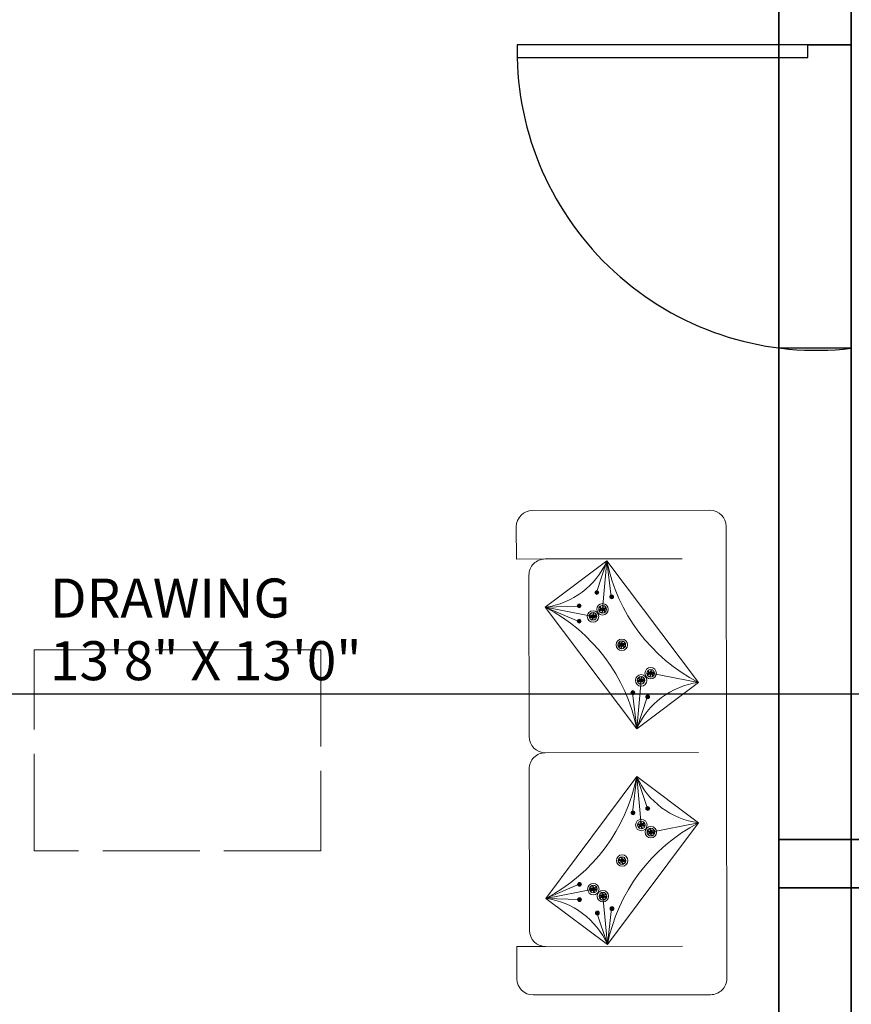
# Model space of a CAD drawing. Units: inches. Extents: x -61 to 1599, y -1316 to 257.
# Tile 30 of 204: x 442 to 545, y -912 to -790. Entities that reach past the tile are written whole.
import ezdxf

# ---------------------------------------------------------------- set-up
doc = ezdxf.new("R2010")
doc.units = ezdxf.units.IN
doc.header["$MEASUREMENT"] = 0
doc.linetypes.add('ACAD_ISO02W100', pattern=[15, 12, -3])
for name, color, linetype, lineweight in [('A-ANNO-DIMS', 2, 'Continuous', 18), ('A-AREA-IDEN', 1, 'Continuous', 18), ('A-FURN-LOW', 83, 'ACAD_ISO02W100', 18), ('A-WALL-JAMB', 4, 'ACAD_ISO02W100', 25), ('DOORS', 2, 'Continuous', 25), ('FURNITURE', 83, 'Continuous', 18), ('WALLS', 4, 'Continuous', 35)]:
    doc.layers.add(name, color=color, linetype=linetype, lineweight=lineweight)
doc.layers.add('FUR', color=83, linetype='Continuous')
doc.styles.get("Standard").update_dxf_attribs({"font": 'arial.ttf'})
doc.dimstyles.get("Standard").update_dxf_attribs({"dimtxt": 0.18, "dimasz": 0.18, "dimexe": 0.18, "dimexo": 0.0625, "dimgap": 0.09, "dimtad": 0, "dimtih": 1, "dimtoh": 1, "dimdec": 0, "dimzin": 0, "dimdsep": 46, "dimlunit": 3, "dimtxsty": 'Standard', "dimcen": 0.09, "dimadec": 0, "dimazin": 0, "dimtfac": 1, "dimtdec": 0, "dimtofl": 0, "dimtmove": 0, "dimatfit": 3, "dimfxl": 1, "dimtolj": 1, "dimtzin": 0, "dimarcsym": 0})

# ---------------------------------------------------------------- blocks, each defined once
blk = doc.blocks.new('*U382')
at = {"layer": 'FUR'}
blk.add_open_spline([(0.01, 0.24), (-0.09, 0.14), (-0.29, -0.05), (0.22, -0.05), (0.07, -0.19), (0.01, -0.24)], degree=3, knots=[0, 0, 0, 0, 0.2846533, 0.5662105, 0.736751, 0.736751, 0.736751, 0.736751], dxfattribs=at)
blk = doc.blocks.new('*U383')
at = {"layer": 'FURNITURE', "transparency": 16777216}
for p, rotation in [((662.52, -238.49), 60), ((662.53, -238.73), 120), ((662.74, -238.83), 180), ((662.93, -238.46), 300), ((662.94, -238.7), 240)]:
    blk.add_blockref('*U382', p, dxfattribs=dict(at, rotation=rotation))
blk.add_blockref('*U382', (662.72, -238.36), dxfattribs=at)
blk = doc.blocks.new('*U394')
at = {"layer": 'FUR'}
blk.add_open_spline([(0.01, 0.24), (-0.09, 0.14), (-0.29, -0.05), (0.22, -0.05), (0.07, -0.19), (0.01, -0.24)], degree=3, knots=[0, 0, 0, 0, 0.2846533, 0.5662105, 0.736751, 0.736751, 0.736751, 0.736751], dxfattribs=at)
blk = doc.blocks.new('*U411')
at = {"layer": 'FURNITURE', "transparency": 16777216}
for p, rotation in [((662.52, -238.49), 60), ((662.53, -238.73), 120), ((662.74, -238.83), 180), ((662.93, -238.46), 300), ((662.94, -238.7), 240)]:
    blk.add_blockref('*U394', p, dxfattribs=dict(at, rotation=rotation))
blk.add_blockref('*U394', (662.72, -238.36), dxfattribs=at)
blk = doc.blocks.new('*U384')
at = {"layer": 'FUR'}
blk.add_open_spline([(0, 0.08), (-0.03, 0.05), (-0.1, -0.02), (0.08, -0.02), (0.02, -0.06), (0, -0.08)], degree=3, knots=[0, 0, 0, 0, 0.0954578, 0.1898773, 0.2470677, 0.2470677, 0.2470677, 0.2470677], dxfattribs=at)
blk = doc.blocks.new('*U385')
at = {"layer": 'FURNITURE', "transparency": 16777216}
for p, rotation in [((222.17, -79.98), 60), ((222.18, -80.06), 120), ((222.31, -79.97), 300), ((222.25, -80.09), 180), ((222.32, -80.05), 240)]:
    blk.add_blockref('*U384', p, dxfattribs=dict(at, rotation=rotation))
blk.add_blockref('*U384', (222.24, -79.93), dxfattribs=at)
blk = doc.blocks.new('*U386')
at = {"layer": 'FUR'}
blk.add_open_spline([(0, 0.08), (-0.03, 0.05), (-0.1, -0.02), (0.08, -0.02), (0.02, -0.06), (0, -0.08)], degree=3, knots=[0, 0, 0, 0, 0.0954578, 0.1898773, 0.2470677, 0.2470677, 0.2470677, 0.2470677], dxfattribs=at)
blk = doc.blocks.new('*U387')
at = {"layer": 'FURNITURE', "transparency": 16777216}
for p, rotation in [((222.17, -79.98), 60), ((222.18, -80.06), 120), ((222.31, -79.97), 300), ((222.25, -80.09), 180), ((222.32, -80.05), 240)]:
    blk.add_blockref('*U386', p, dxfattribs=dict(at, rotation=rotation))
blk.add_blockref('*U386', (222.24, -79.93), dxfattribs=at)
blk = doc.blocks.new('*U388')
at = {"layer": 'FUR'}
blk.add_open_spline([(0, 0.08), (-0.03, 0.05), (-0.1, -0.02), (0.08, -0.02), (0.02, -0.06), (0, -0.08)], degree=3, knots=[0, 0, 0, 0, 0.0954578, 0.1898773, 0.2470677, 0.2470677, 0.2470677, 0.2470677], dxfattribs=at)
blk = doc.blocks.new('*U389')
at = {"layer": 'FURNITURE', "transparency": 16777216}
for p, rotation in [((222.17, -79.98), 60), ((222.18, -80.06), 120), ((222.31, -79.97), 300), ((222.25, -80.09), 180), ((222.32, -80.05), 240)]:
    blk.add_blockref('*U388', p, dxfattribs=dict(at, rotation=rotation))
blk.add_blockref('*U388', (222.24, -79.93), dxfattribs=at)
blk = doc.blocks.new('*U390')
at = {"layer": 'FUR'}
blk.add_open_spline([(0, 0.08), (-0.03, 0.05), (-0.1, -0.02), (0.08, -0.02), (0.02, -0.06), (0, -0.08)], degree=3, knots=[0, 0, 0, 0, 0.0954578, 0.1898773, 0.2470677, 0.2470677, 0.2470677, 0.2470677], dxfattribs=at)
blk = doc.blocks.new('*U391')
at = {"layer": 'FURNITURE', "transparency": 16777216}
for p, rotation in [((222.17, -79.98), 60), ((222.18, -80.06), 120), ((222.31, -79.97), 300), ((222.25, -80.09), 180), ((222.32, -80.05), 240)]:
    blk.add_blockref('*U390', p, dxfattribs=dict(at, rotation=rotation))
blk.add_blockref('*U390', (222.24, -79.93), dxfattribs=at)
blk = doc.blocks.new('*U392')
at = {"layer": 'FUR'}
blk.add_open_spline([(0, 0.08), (-0.03, 0.05), (-0.1, -0.02), (0.08, -0.02), (0.02, -0.06), (0, -0.08)], degree=3, knots=[0, 0, 0, 0, 0.0954578, 0.1898773, 0.2470677, 0.2470677, 0.2470677, 0.2470677], dxfattribs=at)
blk = doc.blocks.new('*U413')
at = {"layer": 'FURNITURE', "transparency": 16777216}
for p, rotation in [((222.17, -79.98), 60), ((222.18, -80.06), 120), ((222.31, -79.97), 300), ((222.25, -80.09), 180), ((222.32, -80.05), 240)]:
    blk.add_blockref('*U392', p, dxfattribs=dict(at, rotation=rotation))
blk.add_blockref('*U392', (222.24, -79.93), dxfattribs=at)
blk = doc.blocks.new('*U414')
at = {"layer": 'FUR'}
blk.add_open_spline([(0, 0.08), (-0.03, 0.05), (-0.1, -0.02), (0.08, -0.02), (0.02, -0.06), (0, -0.08)], degree=3, knots=[0, 0, 0, 0, 0.0954578, 0.1898773, 0.2470677, 0.2470677, 0.2470677, 0.2470677], dxfattribs=at)
blk = doc.blocks.new('*U415')
at = {"layer": 'FURNITURE', "transparency": 16777216}
for p, rotation in [((222.17, -79.98), 60), ((222.18, -80.06), 120), ((222.31, -79.97), 300), ((222.25, -80.09), 180), ((222.32, -80.05), 240)]:
    blk.add_blockref('*U414', p, dxfattribs=dict(at, rotation=rotation))
blk.add_blockref('*U414', (222.24, -79.93), dxfattribs=at)
blk = doc.blocks.new('*U416')
at = {"layer": 'FUR'}
blk.add_open_spline([(0.01, 0.24), (-0.09, 0.14), (-0.29, -0.05), (0.22, -0.05), (0.07, -0.19), (0.01, -0.24)], degree=3, knots=[0, 0, 0, 0, 0.2846533, 0.5662105, 0.736751, 0.736751, 0.736751, 0.736751], dxfattribs=at)
blk = doc.blocks.new('*U417')
at = {"layer": 'FURNITURE', "transparency": 16777216}
for p, rotation in [((662.52, -238.49), 60), ((662.53, -238.73), 120), ((662.74, -238.83), 180), ((662.93, -238.46), 300), ((662.94, -238.7), 240)]:
    blk.add_blockref('*U416', p, dxfattribs=dict(at, rotation=rotation))
blk.add_blockref('*U416', (662.72, -238.36), dxfattribs=at)
blk = doc.blocks.new('*U418')
at = {"layer": 'FUR'}
blk.add_open_spline([(0.01, 0.24), (-0.09, 0.14), (-0.29, -0.05), (0.22, -0.05), (0.07, -0.19), (0.01, -0.24)], degree=3, knots=[0, 0, 0, 0, 0.2846533, 0.5662105, 0.736751, 0.736751, 0.736751, 0.736751], dxfattribs=at)
blk = doc.blocks.new('*U381')
at = {"layer": 'FURNITURE', "transparency": 16777216}
for p, rotation in [((662.52, -238.49), 60), ((662.53, -238.73), 120), ((662.74, -238.83), 180), ((662.93, -238.46), 300), ((662.94, -238.7), 240)]:
    blk.add_blockref('*U418', p, dxfattribs=dict(at, rotation=rotation))
blk.add_blockref('*U418', (662.72, -238.36), dxfattribs=at)
blk = doc.blocks.new('*U393')
at = {"layer": 'FUR'}
blk.add_open_spline([(0.01, 0.24), (-0.09, 0.14), (-0.29, -0.05), (0.22, -0.05), (0.07, -0.19), (0.01, -0.24)], degree=3, knots=[0, 0, 0, 0, 0.2846533, 0.5662105, 0.736751, 0.736751, 0.736751, 0.736751], dxfattribs=at)
blk = doc.blocks.new('*U412')
at = {"layer": 'FURNITURE', "transparency": 16777216}
for p, rotation in [((662.52, -238.49), 60), ((662.53, -238.73), 120), ((662.74, -238.83), 180), ((662.93, -238.46), 300), ((662.94, -238.7), 240)]:
    blk.add_blockref('*U393', p, dxfattribs=dict(at, rotation=rotation))
blk.add_blockref('*U393', (662.72, -238.36), dxfattribs=at)
blk = doc.blocks.new('*U379')
at = {"layer": 'FUR'}
blk.add_open_spline([(0.01, 0.24), (-0.09, 0.14), (-0.29, -0.05), (0.22, -0.05), (0.07, -0.19), (0.01, -0.24)], degree=3, knots=[0, 0, 0, 0, 0.2846533, 0.5662105, 0.736751, 0.736751, 0.736751, 0.736751], dxfattribs=at)
blk = doc.blocks.new('*U380')
at = {"layer": 'FURNITURE', "transparency": 16777216}
for p, rotation in [((662.52, -238.49), 60), ((662.53, -238.73), 120), ((662.74, -238.83), 180), ((662.93, -238.46), 300), ((662.94, -238.7), 240)]:
    blk.add_blockref('*U379', p, dxfattribs=dict(at, rotation=rotation))
blk.add_blockref('*U379', (662.72, -238.36), dxfattribs=at)
blk = doc.blocks.new('*U410')
at = {"layer": 'FUR'}
blk.add_open_spline([(0.01, 0.24), (-0.09, 0.14), (-0.29, -0.05), (0.22, -0.05), (0.07, -0.19), (0.01, -0.24)], degree=3, knots=[0, 0, 0, 0, 0.2846533, 0.5662105, 0.736751, 0.736751, 0.736751, 0.736751], dxfattribs=at)
blk = doc.blocks.new('*U395')
at = {"layer": 'FURNITURE', "transparency": 16777216}
for p, rotation in [((662.52, -238.49), 60), ((662.53, -238.73), 120), ((662.74, -238.83), 180), ((662.93, -238.46), 300), ((662.94, -238.7), 240)]:
    blk.add_blockref('*U410', p, dxfattribs=dict(at, rotation=rotation))
blk.add_blockref('*U410', (662.72, -238.36), dxfattribs=at)
blk = doc.blocks.new('*U400')
at = {"layer": 'FUR'}
blk.add_open_spline([(0, 0.08), (-0.03, 0.05), (-0.1, -0.02), (0.08, -0.02), (0.02, -0.06), (0, -0.08)], degree=3, knots=[0, 0, 0, 0, 0.0954578, 0.1898773, 0.2470677, 0.2470677, 0.2470677, 0.2470677], dxfattribs=at)
blk = doc.blocks.new('*U401')
at = {"layer": 'FURNITURE', "transparency": 16777216}
for p, rotation in [((222.17, -79.98), 60), ((222.18, -80.06), 120), ((222.31, -79.97), 300), ((222.25, -80.09), 180), ((222.32, -80.05), 240)]:
    blk.add_blockref('*U400', p, dxfattribs=dict(at, rotation=rotation))
blk.add_blockref('*U400', (222.24, -79.93), dxfattribs=at)
blk = doc.blocks.new('*U402')
at = {"layer": 'FUR'}
blk.add_open_spline([(0, 0.08), (-0.03, 0.05), (-0.1, -0.02), (0.08, -0.02), (0.02, -0.06), (0, -0.08)], degree=3, knots=[0, 0, 0, 0, 0.0954578, 0.1898773, 0.2470677, 0.2470677, 0.2470677, 0.2470677], dxfattribs=at)
blk = doc.blocks.new('*U403')
at = {"layer": 'FURNITURE', "transparency": 16777216}
for p, rotation in [((222.17, -79.98), 60), ((222.18, -80.06), 120), ((222.31, -79.97), 300), ((222.25, -80.09), 180), ((222.32, -80.05), 240)]:
    blk.add_blockref('*U402', p, dxfattribs=dict(at, rotation=rotation))
blk.add_blockref('*U402', (222.24, -79.93), dxfattribs=at)
blk = doc.blocks.new('*U404')
at = {"layer": 'FUR'}
blk.add_open_spline([(0, 0.08), (-0.03, 0.05), (-0.1, -0.02), (0.08, -0.02), (0.02, -0.06), (0, -0.08)], degree=3, knots=[0, 0, 0, 0, 0.0954578, 0.1898773, 0.2470677, 0.2470677, 0.2470677, 0.2470677], dxfattribs=at)
blk = doc.blocks.new('*U405')
at = {"layer": 'FURNITURE', "transparency": 16777216}
for p, rotation in [((222.17, -79.98), 60), ((222.18, -80.06), 120), ((222.31, -79.97), 300), ((222.25, -80.09), 180), ((222.32, -80.05), 240)]:
    blk.add_blockref('*U404', p, dxfattribs=dict(at, rotation=rotation))
blk.add_blockref('*U404', (222.24, -79.93), dxfattribs=at)
blk = doc.blocks.new('*U406')
at = {"layer": 'FUR'}
blk.add_open_spline([(0, 0.08), (-0.03, 0.05), (-0.1, -0.02), (0.08, -0.02), (0.02, -0.06), (0, -0.08)], degree=3, knots=[0, 0, 0, 0, 0.0954578, 0.1898773, 0.2470677, 0.2470677, 0.2470677, 0.2470677], dxfattribs=at)
blk = doc.blocks.new('*U407')
at = {"layer": 'FURNITURE', "transparency": 16777216}
for p, rotation in [((222.17, -79.98), 60), ((222.18, -80.06), 120), ((222.31, -79.97), 300), ((222.25, -80.09), 180), ((222.32, -80.05), 240)]:
    blk.add_blockref('*U406', p, dxfattribs=dict(at, rotation=rotation))
blk.add_blockref('*U406', (222.24, -79.93), dxfattribs=at)
blk = doc.blocks.new('*U408')
at = {"layer": 'FUR'}
blk.add_open_spline([(0, 0.08), (-0.03, 0.05), (-0.1, -0.02), (0.08, -0.02), (0.02, -0.06), (0, -0.08)], degree=3, knots=[0, 0, 0, 0, 0.0954578, 0.1898773, 0.2470677, 0.2470677, 0.2470677, 0.2470677], dxfattribs=at)
blk = doc.blocks.new('*U397')
at = {"layer": 'FURNITURE', "transparency": 16777216}
for p, rotation in [((222.17, -79.98), 60), ((222.18, -80.06), 120), ((222.31, -79.97), 300), ((222.25, -80.09), 180), ((222.32, -80.05), 240)]:
    blk.add_blockref('*U408', p, dxfattribs=dict(at, rotation=rotation))
blk.add_blockref('*U408', (222.24, -79.93), dxfattribs=at)
blk = doc.blocks.new('*U398')
at = {"layer": 'FUR'}
blk.add_open_spline([(0, 0.08), (-0.03, 0.05), (-0.1, -0.02), (0.08, -0.02), (0.02, -0.06), (0, -0.08)], degree=3, knots=[0, 0, 0, 0, 0.0954578, 0.1898773, 0.2470677, 0.2470677, 0.2470677, 0.2470677], dxfattribs=at)
blk = doc.blocks.new('*U399')
at = {"layer": 'FURNITURE', "transparency": 16777216}
for p, rotation in [((222.17, -79.98), 60), ((222.18, -80.06), 120), ((222.31, -79.97), 300), ((222.25, -80.09), 180), ((222.32, -80.05), 240)]:
    blk.add_blockref('*U398', p, dxfattribs=dict(at, rotation=rotation))
blk.add_blockref('*U398', (222.24, -79.93), dxfattribs=at)
blk = doc.blocks.new('*U375')
at = {"layer": 'FUR'}
blk.add_open_spline([(0.01, 0.24), (-0.09, 0.14), (-0.29, -0.05), (0.22, -0.05), (0.07, -0.19), (0.01, -0.24)], degree=3, knots=[0, 0, 0, 0, 0.2846533, 0.5662105, 0.736751, 0.736751, 0.736751, 0.736751], dxfattribs=at)
blk = doc.blocks.new('*U376')
at = {"layer": 'FURNITURE', "transparency": 16777216}
for p, rotation in [((662.52, -238.49), 60), ((662.53, -238.73), 120), ((662.74, -238.83), 180), ((662.93, -238.46), 300), ((662.94, -238.7), 240)]:
    blk.add_blockref('*U375', p, dxfattribs=dict(at, rotation=rotation))
blk.add_blockref('*U375', (662.72, -238.36), dxfattribs=at)
blk = doc.blocks.new('*U377')
at = {"layer": 'FUR'}
blk.add_open_spline([(0.01, 0.24), (-0.09, 0.14), (-0.29, -0.05), (0.22, -0.05), (0.07, -0.19), (0.01, -0.24)], degree=3, knots=[0, 0, 0, 0, 0.2846533, 0.5662105, 0.736751, 0.736751, 0.736751, 0.736751], dxfattribs=at)
blk = doc.blocks.new('*U378')
at = {"layer": 'FURNITURE', "transparency": 16777216}
for p, rotation in [((662.52, -238.49), 60), ((662.53, -238.73), 120), ((662.74, -238.83), 180), ((662.93, -238.46), 300), ((662.94, -238.7), 240)]:
    blk.add_blockref('*U377', p, dxfattribs=dict(at, rotation=rotation))
blk.add_blockref('*U377', (662.72, -238.36), dxfattribs=at)
blk = doc.blocks.new('*U409')
at = {"layer": 'FUR'}
blk.add_open_spline([(0.01, 0.24), (-0.09, 0.14), (-0.29, -0.05), (0.22, -0.05), (0.07, -0.19), (0.01, -0.24)], degree=3, knots=[0, 0, 0, 0, 0.2846533, 0.5662105, 0.736751, 0.736751, 0.736751, 0.736751], dxfattribs=at)
blk = doc.blocks.new('*U396')
at = {"layer": 'FURNITURE', "transparency": 16777216}
for p, rotation in [((662.52, -238.49), 60), ((662.53, -238.73), 120), ((662.74, -238.83), 180), ((662.93, -238.46), 300), ((662.94, -238.7), 240)]:
    blk.add_blockref('*U409', p, dxfattribs=dict(at, rotation=rotation))
blk.add_blockref('*U409', (662.72, -238.36), dxfattribs=at)
blk = doc.blocks.new('DOOR-SWING-36')
blk.add_line((0, 0), (0, -5.4))
blk.add_lwpolyline([(0, 0), (0, 36), (-1.57, 36), (-1.57, 0)], close=True)
blk.add_arc((-0.74, -1.08), 37.09, 91.2913, 186.6905)
blk = doc.blocks.new('*D696')
at = {"layer": 'A-ANNO-DIMS', "color": 0, "lineweight": -2, "transparency": 16777216}
for p, q in [((690.64, -873.17), (-61.08, -873.17)), ((-60.9, -873.35), (-60.9, -1025.8)), ((-60.9, -1178.61), (-60.9, -1026.16)), ((690.64, -1178.79), (-61.08, -1178.79))]:
    blk.add_line(p, q, dxfattribs=at)
at = {"layer": 'A-ANNO-DIMS', "color": 0, "transparency": 16777216}
for points in [[(-60.93, -873.35), (-60.87, -873.35), (-60.9, -873.17)], [(-60.93, -1178.61), (-60.87, -1178.61), (-60.9, -1178.79)]]:
    blk.add_solid(points, dxfattribs=at)
at = {"layer": 'DEFPOINTS', "color": 0, "transparency": 16777216}
for p in [(-60.9, -873.17), (690.7, -873.17), (690.7, -1178.79)]:
    blk.add_point(p, dxfattribs=at)
at = {"layer": 'A-ANNO-DIMS', "color": 0, "transparency": 16777216, "insert": (-60.9, -1025.98), "char_height": 0.18, "attachment_point": 5}
blk.add_mtext('\\A1;305.6', dxfattribs=at)

msp = doc.modelspace()

# ---------------------------------------------------------------- linework, layer by layer
at = {"layer": 'A-FURN-LOW'}
msp.add_lwpolyline([(478.9662, -892.5776), (443.4644, -892.5776), (443.4644, -867.6738), (478.9662, -867.6738)], close=True, dxfattribs=at)
at = {"layer": 'A-WALL-JAMB'}
for p, q in [((544.7028, -792.7635), (535.7028, -792.7635)), ((544.7028, -830.3385), (535.7028, -830.3385))]:
    msp.add_line(p, q, dxfattribs=at)
at = {"layer": 'FURNITURE'}
for p, q in [((506.7579, -856.4365), (503.1999, -856.4414)), ((506.7579, -856.4365), (523.7299, -856.4132)), ((514.4247, -856.6747), (513.1247, -860.6102)), ((514.4247, -856.6747), (513.8773, -862.6696)), ((514.4247, -856.6747), (514.9538, -861.1398)), ((504.7607, -858.4393), (504.7882, -878.4393)), ((513.1772, -860.5908), (513.0174, -860.591)), ((513.1772, -860.5908), (513.337, -860.5905)), ((506.7866, -862.4232), (510.9281, -862.2634)), ((510.9805, -862.244), (510.8207, -862.2442)), ((510.9805, -862.244), (511.1403, -862.2437)), ((515.0062, -861.1203), (514.8464, -861.1206)), ((515.0062, -861.1203), (515.166, -861.1201)), ((506.7866, -862.4232), (512.6987, -863.5566)), ((506.7866, -862.4232), (510.9307, -864.1675)), ((513.8773, -862.6696), (513.4008, -862.6702)), ((513.8773, -862.6696), (514.3538, -862.6689)), ((510.9831, -864.1481), (510.8233, -864.1483)), ((510.9831, -864.1481), (511.1429, -864.1479)), ((512.6987, -863.5566), (512.2222, -863.5572)), ((512.6987, -863.5566), (513.1752, -863.5559)), ((516.2688, -867.0737), (515.7923, -867.0744)), ((516.2688, -867.0737), (516.7452, -867.073)), ((519.8388, -870.5908), (519.3623, -870.5915)), ((519.8388, -870.5908), (520.3153, -870.5902)), ((525.7509, -871.7242), (519.8388, -870.5908)), ((518.1128, -877.4727), (518.6602, -871.4778)), ((518.6602, -871.4778), (518.1837, -871.4785)), ((518.6602, -871.4778), (519.1367, -871.4772)), ((517.6362, -872.9882), (517.4764, -872.9884)), ((518.1128, -877.4727), (517.5838, -873.0076)), ((517.6362, -872.9882), (517.796, -872.988)), ((518.1128, -877.4727), (519.4128, -873.5372)), ((519.4652, -873.5178), (519.3054, -873.518)), ((519.4652, -873.5178), (519.625, -873.5176)), ((506.7909, -880.4365), (525.7629, -880.4105)), ((506.7909, -880.4365), (506.7909, -880.4365)), ((504.8212, -902.4393), (504.7937, -882.4393)), ((518.121, -883.395), (517.6042, -887.8614)), ((518.121, -883.395), (518.6848, -889.3882)), ((518.121, -883.395), (519.4317, -887.3268)), ((517.6567, -887.8807), (517.4969, -887.8809)), ((517.6567, -887.8807), (517.8165, -887.8805)), ((519.4842, -887.3461), (519.3244, -887.3463)), ((519.4842, -887.3461), (519.644, -887.3459)), ((518.6848, -889.3882), (518.2084, -889.3889)), ((518.6848, -889.3882), (519.1613, -889.3876)), ((519.8659, -890.272), (519.3894, -890.2727)), ((525.7748, -889.1224), (519.8659, -890.272)), ((519.8659, -890.272), (520.3424, -890.2714)), ((516.3055, -893.7989), (515.829, -893.7996)), ((516.3055, -893.7989), (516.782, -893.7983)), ((506.8361, -898.4755), (510.9754, -896.7198)), ((506.8361, -898.4755), (512.7451, -897.3259)), ((511.0279, -896.7391), (510.8681, -896.7393)), ((511.0279, -896.7391), (511.1877, -896.7388)), ((512.7451, -897.3259), (512.2686, -897.3265)), ((512.7451, -897.3259), (513.2216, -897.3252)), ((506.8361, -898.4755), (510.978, -898.6239)), ((511.0305, -898.6432), (510.8708, -898.6434)), ((511.0305, -898.6432), (511.1903, -898.643)), ((513.9261, -898.2096), (513.4496, -898.2103)), ((513.9261, -898.2096), (514.4026, -898.209)), ((514.49, -904.2029), (513.9261, -898.2096)), ((514.49, -904.2029), (515.0068, -899.7365)), ((515.0593, -899.7557), (514.8995, -899.756)), ((515.0593, -899.7557), (515.2191, -899.7555)), ((513.2318, -900.2904), (513.072, -900.2906)), ((514.49, -904.2029), (513.1793, -900.2711)), ((513.2318, -900.2904), (513.3915, -900.2901)), ((506.8239, -904.4365), (503.2659, -904.4414)), ((506.8239, -904.4365), (523.7958, -904.4132))]:
    msp.add_line(p, q, dxfattribs=at)
msp.add_lwpolyline([(503.2659, -904.4414), (503.2714, -908.4414, 0.41421356), (505.2742, -910.4387), (527.2741, -910.4084, 0.41421369), (529.2714, -908.4057), (529.1944, -852.4057, 0.41421343), (527.1916, -850.4084), (505.1917, -850.4387, 0.41421356), (503.1944, -852.4414), (503.1999, -856.4414)], format="xyb", dxfattribs=at)
for points in [[(518.1128, -877.4727), (506.7866, -862.4232), (514.4247, -856.6747), (525.7509, -871.7242)], [(518.121, -883.395), (506.8361, -898.4755), (514.49, -904.2029), (525.7748, -889.1224)]]:
    msp.add_lwpolyline(points, close=True, dxfattribs=at)
for centre, radius in [((513.1772, -860.5908), 0.2382), ((513.1772, -860.5908), 0.1598), ((515.0062, -861.1203), 0.2382), ((515.0062, -861.1203), 0.1598), ((510.9805, -862.244), 0.2382), ((510.9805, -862.244), 0.1598), ((513.8773, -862.6696), 0.7104), ((513.8773, -862.6696), 0.4765), ((512.6987, -863.5566), 0.7104), ((512.6987, -863.5566), 0.4765), ((510.9831, -864.1481), 0.2382), ((510.9831, -864.1481), 0.1598), ((516.2688, -867.0737), 0.7104), ((516.2688, -867.0737), 0.4765), ((518.6602, -871.4778), 0.7104), ((519.8388, -870.5908), 0.7104), ((519.8388, -870.5908), 0.4765), ((518.6602, -871.4778), 0.4765), ((517.6362, -872.9882), 0.2382), ((517.6362, -872.9882), 0.1598), ((519.4652, -873.5178), 0.2382), ((519.4652, -873.5178), 0.1598), ((517.6567, -887.8807), 0.2382), ((517.6567, -887.8807), 0.1598), ((519.4842, -887.3461), 0.2382), ((519.4842, -887.3461), 0.1598), ((518.6848, -889.3882), 0.7104), ((518.6848, -889.3882), 0.4765), ((519.8659, -890.272), 0.7104), ((519.8659, -890.272), 0.4765), ((516.3055, -893.7989), 0.7104), ((516.3055, -893.7989), 0.4765), ((511.0279, -896.7391), 0.2382), ((511.0279, -896.7391), 0.1598), ((512.7451, -897.3259), 0.7104), ((512.7451, -897.3259), 0.4765), ((513.9261, -898.2096), 0.7104), ((511.0305, -898.6432), 0.2382), ((511.0305, -898.6432), 0.1598), ((513.9261, -898.2096), 0.4765), ((513.2318, -900.2904), 0.2382), ((515.0593, -899.7557), 0.2382), ((515.0593, -899.7557), 0.1598), ((513.2318, -900.2904), 0.1598)]:
    msp.add_circle(centre, radius, dxfattribs=at)
for centre, radius, start, end in [((506.7607, -858.4365), 2, 90.078764, 180.078764), ((505.45, -852.6986), 9.816, 277.825767, 336.104516), ((535.7357, -852.4229), 21.731, 191.283178, 242.647105), ((496.8019, -881.7245), 21.731, 11.283178, 62.647105), ((527.0875, -881.4488), 9.816, 97.825767, 156.104516), ((506.7882, -878.4366), 2, 180.078764, 270.078764), ((506.7937, -882.4365), 2, 90.078764, 180.078764), ((496.7984, -879.2017), 21.731, 297.510392, 348.87432), ((527.0847, -879.3941), 9.816, 204.052981, 262.33173), ((535.8126, -908.3962), 21.731, 117.510392, 168.87432), ((505.5263, -908.2037), 9.816, 24.052981, 82.33173), ((506.8212, -902.4365), 2, 180.078764, 270.078764)]:
    msp.add_arc(centre, radius, start, end, dxfattribs=at)
at = {"layer": 'WALLS'}
for p, q in [((535.7028, -1215.9446), (535.7028, -741.169)), ((544.7028, -1215.9446), (544.7028, -741.169)), ((535.7028, -891.169), (690.7028, -891.169)), ((535.7028, -897.169), (690.7028, -897.169))]:
    msp.add_line(p, q, dxfattribs=at)

# ---------------------------------------------------------------- block references
at = {"layer": 'DOORS', "rotation": 89.99999999999297}
msp.add_blockref('DOOR-SWING-36', (539.3028, -792.7635), dxfattribs=at)
at = {"layer": 'FURNITURE', "rotation": 270.0787336990067}
for name, p in [('*U397', (592.884, -638.2361)), ('*U399', (594.713, -638.7657)), ('*U405', (590.6874, -639.8893)), ('*U396', (751.5615, -199.6122)), ('*U376', (750.383, -200.4992)), ('*U407', (590.69, -641.7934)), ('*U380', (753.953, -204.0163)), ('*U395', (757.5231, -207.5335)), ('*U378', (756.3445, -208.4205)), ('*U403', (597.343, -650.6335)), ('*U401', (599.1721, -651.1631))]:
    msp.add_blockref(name, p, dxfattribs=at)
at = {"layer": 'FURNITURE', "xscale": -1, "rotation": 270.0787636990076}
for name, p in [('*U387', (597.9744, -1110.0154)), ('*U385', (599.802, -1109.4808)), ('*U381', (758.1909, -1551.7898)), ('*U411', (759.3719, -1552.6735)), ('*U383', (755.8115, -1556.2004)), ('*U391', (591.3457, -1118.8738)), ('*U417', (752.2511, -1559.7274)), ('*U389', (591.3483, -1120.7779)), ('*U412', (753.4321, -1560.6111)), ('*U415', (595.3771, -1121.8905)), ('*U413', (593.5495, -1122.4251))]:
    msp.add_blockref(name, p, dxfattribs=at)

# ---------------------------------------------------------------- texts
at = {"layer": 'A-AREA-IDEN'}
for s, height, p in [('DRAWING', 4.8321, (445.4206, -863.6909)), ('13\'8" X 13\'0"', 4.832098, (445.4206, -871.4532))]:
    msp.add_text(s, height=height, dxfattribs=at).set_placement(p)

# ---------------------------------------------------------------- dimensions: what is measured, and where the dimension line sits
at = {"layer": 'A-ANNO-DIMS'}
dim = msp.add_linear_dim(base=(-60.8972, -873.169), p1=(690.7028, -1178.7933), p2=(690.7028, -873.169), angle=90, dimstyle='Standard', override={"dimdec": 1, "dimlfac": 1, "dimrnd": 0, "dimzin": 0, "dimdsep": 46, "dimlunit": 2}, dxfattribs=at)
dim.commit()
dim.dimension.update_dxf_attribs({"geometry": '*D696', "text_midpoint": (-60.8972, -1025.9812)})

doc.saveas('drawing.dxf')
